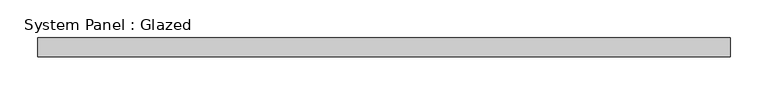
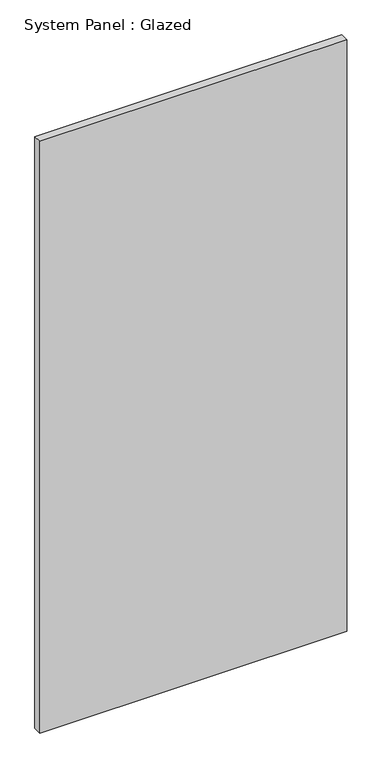
"""IFC4 building model written with IfcOpenShell, lengths in millimetres: plate geometry, System Panel : Glazed."""

from ifc_helpers import new_model, si_unit, origin, origin_with_axes, place, context, project, spatial, polyline, outline, extrude, source, transform, mapped, element, save


def system_panel_glazed_85540d86(model_context):
    return source(origin(), model_context, "Body", "SweptSolid", [
        extrude(outline(polyline([(457.2, 24.5), (-457.2, 24.5), (-457.2, 49.5), (457.2, 49.5), (457.2, 24.5)])), origin_with_axes(), (0.0, 0.0, 1.0), 1864.0),
    ])


if __name__ == "__main__":
    model = new_model("IFC4")
    model_context = context("Model", 3, world=origin())
    ifc_project = project(units=[si_unit("LENGTHUNIT", "METRE", prefix="MILLI")], contexts=[model_context])
    site = spatial("IfcSite", under=ifc_project)
    building = spatial("IfcBuilding", under=site)
    placement = place(None, origin())
    system_panel_glazed_shape = system_panel_glazed_85540d86(model_context)
    element("IfcPlate", 1, ObjectType="System Panel : Glazed", at=placement, inside=building, context=model_context, shape_type="MappedRepresentation", body=[
        mapped(system_panel_glazed_shape, transform((0.0, 0.0, 0.0), x_axis=(1.0, 0.0, 0.0), y_axis=(0.0, 1.0, 0.0), z_axis=(0.0, 0.0, 1.0))),
    ])
    save(model, "model.ifc")

# Revit data of these elements
# Type "System Panel : Glazed"
#   Construction Type Id = "GSP4R"
#   Analytic Construction = "1/8 in Pilkington single glazing"
#   Visual Light Transmittance = 0.9
#   Solar Heat Gain Coefficient = 0.86
#   Heat Transfer Coefficient (U) = 6.7069 W/(m²·K)
#   Define Thermal Properties by = 1
# Element 1 (IfcPlate, "System Panel : Glazed")
#   Materials on its faces: "Glass"
# Materials
#   "Glass": class "Glass", colour RGB 0 128 192, transparency 0.9, Description = "Soda Lime Glass", Cost = 0
